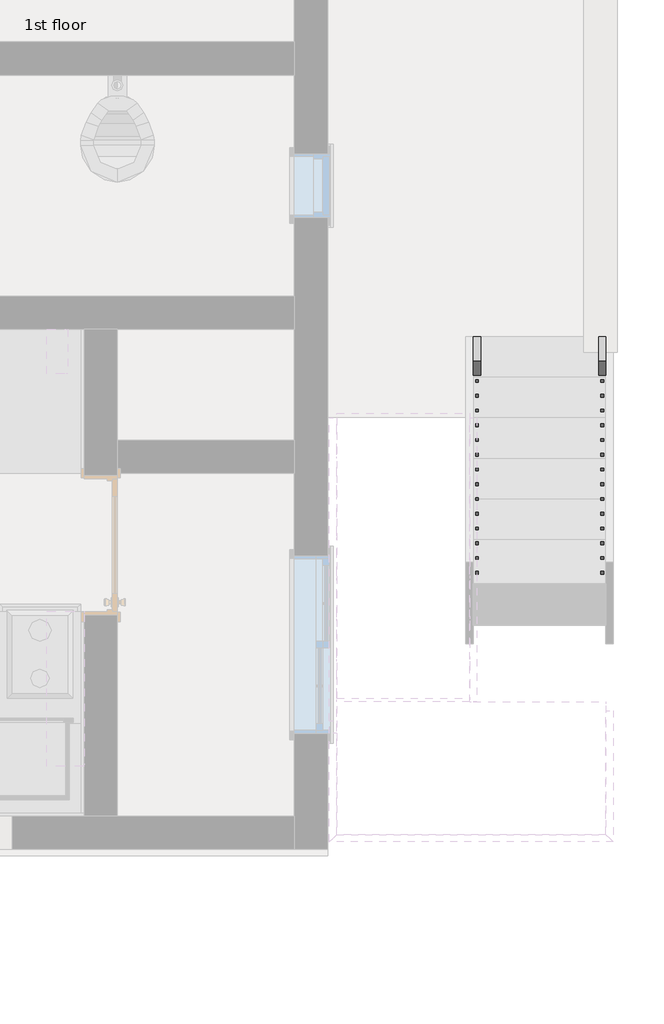
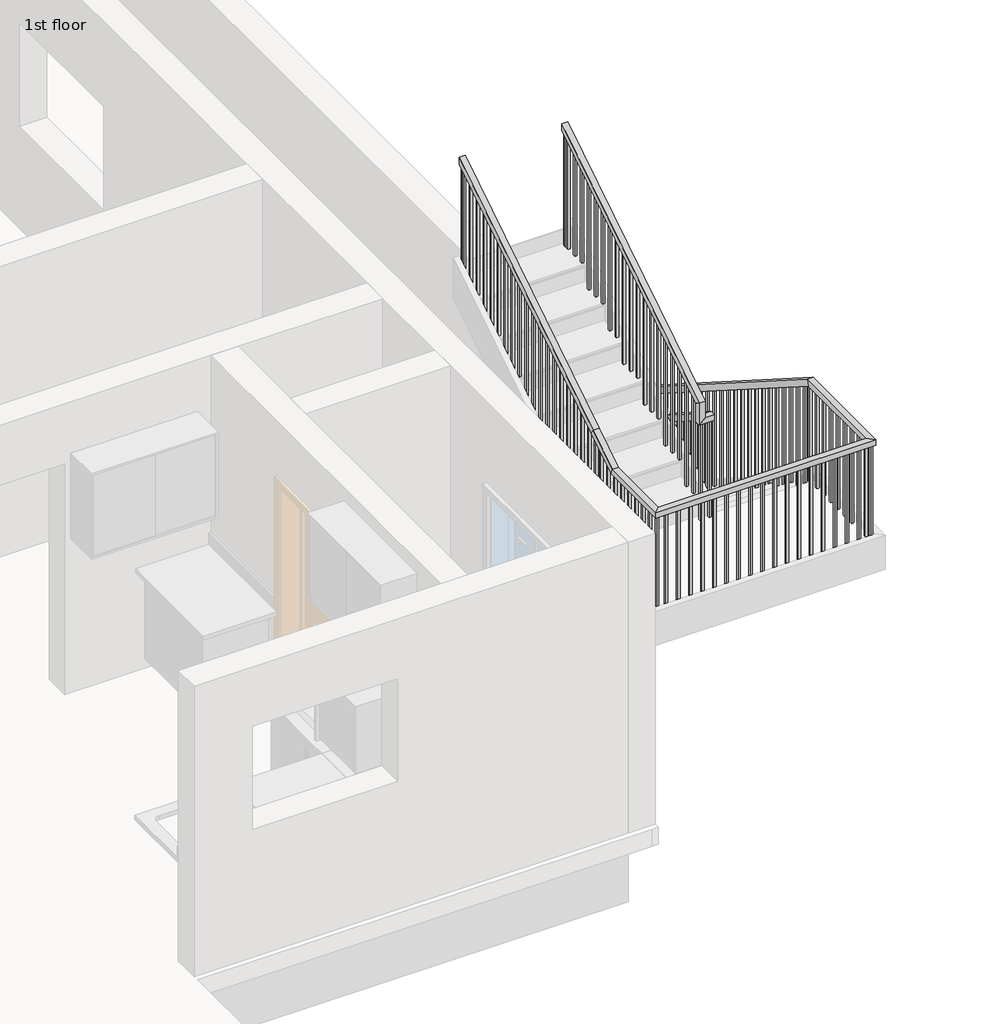
# One storey, part 6 of 8: 2 railings.
"""IFC4 building model written with IfcOpenShell, lengths in millimetres."""

from ifc_helpers import new_model, si_unit, frame, origin, place, context, project, spatial, polyline, outline, extrude, faceted_brep, element, save

model = new_model("IFC4")

# Units and contexts
model_context = context("Model", 3, world=origin())
ifc_project = project(units=[si_unit("LENGTHUNIT", "METRE", prefix="MILLI")], contexts=[model_context])

# Site, building, storey
site = spatial("IfcSite", under=ifc_project)
building = spatial("IfcBuilding", under=site)
storey = spatial("IfcBuildingStorey", under=building, Name="1st floor", Elevation=3810.0)

# Railings
placement = place(None, origin())
element("IfcRailing", 1, ObjectType="Handrail - Rectangular", at=placement, inside=storey, context=model_context, shape_type="SolidModel", body=[
    faceted_brep([(14287.3506237, -1074.7064015, 4902.2), (14287.3506237, -1074.7064015, 4841.986276), (14236.5506237, -1074.7064015, 4841.986276), (14236.5506237, -1074.7064015, 4902.2), (14287.3506237, -3589.3064015, 6502.4), (14236.5506237, -3589.3064015, 6502.4), (14236.5506237, -3589.3064015, 6442.186276), (14287.3506237, -3589.3064015, 6442.186276)], [[[0, 1, 2, 3]], [[4, 5, 6, 7]], [[1, 0, 4, 7]], [[2, 1, 7, 6]], [[3, 2, 6, 5]], [[0, 3, 5, 4]]]),
    faceted_brep([(14287.3506237, -3640.1064015, 6502.4), (14287.3506237, -3640.1064015, 6451.6), (14287.3506237, -3589.3064015, 6451.6), (14287.3506237, -3589.3064015, 6502.4), (14211.1506237, -3640.1064015, 6502.4), (14211.1506237, -3589.3064015, 6502.4), (14160.3506237, -3589.3064015, 6451.6), (14160.3506237, -3640.1064015, 6451.6)], [[[0, 1, 2, 3]], [[4, 5, 6, 7]], [[1, 0, 4, 7]], [[2, 1, 7, 6]], [[3, 2, 6, 5]], [[0, 3, 5, 4]]]),
    faceted_brep([(14211.1506237, -3640.1064015, 6502.4), (14160.3506237, -3640.1064015, 6451.6), (14160.3506237, -3589.3064015, 6451.6), (14211.1506237, -3589.3064015, 6502.4), (14211.1506237, -3640.1064015, 6647.8727273), (14211.1506237, -3589.3064015, 6619.986276), (14160.3506237, -3589.3064015, 6619.986276), (14160.3506237, -3640.1064015, 6647.8727273)], [[[0, 1, 2, 3]], [[4, 5, 6, 7]], [[1, 0, 4, 7]], [[2, 1, 7, 6]], [[3, 2, 6, 5]], [[0, 3, 5, 4]]]),
    faceted_brep([(14160.3506237, -3640.1064015, 6647.8727273), (14160.3506237, -3589.3064015, 6619.986276), (14211.1506237, -3589.3064015, 6619.986276), (14211.1506237, -3640.1064015, 6647.8727273), (14160.3506237, -1633.5064015, 7924.8), (14211.1506237, -1633.5064015, 7924.8), (14211.1506237, -1633.5064015, 7864.586276), (14160.3506237, -1633.5064015, 7864.586276)], [[[0, 1, 2, 3]], [[4, 5, 6, 7]], [[1, 0, 4, 7]], [[2, 1, 7, 6]], [[3, 2, 6, 5]], [[0, 3, 5, 4]]]),
    extrude(outline(polyline([(-1693.8314015, 7826.1976396), (-1674.7814015, 7838.3203669), (-1674.7814015, 6832.6), (-1693.8314015, 6832.6), (-1693.8314015, 7826.1976396)])), frame((14176.2256237, 0.0, 0.0), z_axis=(1.0, 0.0, 0.0), x_axis=(0.0, 1.0, 0.0)), (0.0, 0.0, 1.0), 19.05),
    extrude(outline(polyline([(-1795.4314015, 7761.5430941), (-1776.3814015, 7773.6658214), (-1776.3814015, 6832.6), (-1795.4314015, 6832.6), (-1795.4314015, 7761.5430941)])), frame((14176.2256237, 0.0, 0.0), z_axis=(1.0, 0.0, 0.0), x_axis=(0.0, 1.0, 0.0)), (0.0, 0.0, 1.0), 19.05),
    extrude(outline(polyline([(-1897.0314015, 7696.8885487), (-1877.9814015, 7709.011276), (-1877.9814015, 6832.6), (-1897.0314015, 6832.6), (-1897.0314015, 7696.8885487)])), frame((14176.2256237, 0.0, 0.0), z_axis=(1.0, 0.0, 0.0), x_axis=(0.0, 1.0, 0.0)), (0.0, 0.0, 1.0), 19.05),
    extrude(outline(polyline([(-1998.6314015, 7632.2340032), (-1979.5814015, 7644.3567305), (-1979.5814015, 6654.8), (-1998.6314015, 6654.8), (-1998.6314015, 7632.2340032)])), frame((14176.2256237, 0.0, 0.0), z_axis=(1.0, 0.0, 0.0), x_axis=(0.0, 1.0, 0.0)), (0.0, 0.0, 1.0), 19.05),
    extrude(outline(polyline([(-2100.2314015, 7567.5794578), (-2081.1814015, 7579.7021851), (-2081.1814015, 6654.8), (-2100.2314015, 6654.8), (-2100.2314015, 7567.5794578)])), frame((14176.2256237, 0.0, 0.0), z_axis=(1.0, 0.0, 0.0), x_axis=(0.0, 1.0, 0.0)), (0.0, 0.0, 1.0), 19.05),
    extrude(outline(polyline([(-2201.8314015, 7502.9249123), (-2182.7814015, 7515.0476396), (-2182.7814015, 6654.8), (-2201.8314015, 6654.8), (-2201.8314015, 7502.9249123)])), frame((14176.2256237, 0.0, 0.0), z_axis=(1.0, 0.0, 0.0), x_axis=(0.0, 1.0, 0.0)), (0.0, 0.0, 1.0), 19.05),
    extrude(outline(polyline([(-2303.4314015, 7438.2703669), (-2284.3814015, 7450.3930941), (-2284.3814015, 6477.0), (-2303.4314015, 6477.0), (-2303.4314015, 7438.2703669)])), frame((14176.2256237, 0.0, 0.0), z_axis=(1.0, 0.0, 0.0), x_axis=(0.0, 1.0, 0.0)), (0.0, 0.0, 1.0), 19.05),
    extrude(outline(polyline([(-2405.0314015, 7373.6158214), (-2385.9814015, 7385.7385487), (-2385.9814015, 6477.0), (-2405.0314015, 6477.0), (-2405.0314015, 7373.6158214)])), frame((14176.2256237, 0.0, 0.0), z_axis=(1.0, 0.0, 0.0), x_axis=(0.0, 1.0, 0.0)), (0.0, 0.0, 1.0), 19.05),
    extrude(outline(polyline([(-2506.6314015, 7308.961276), (-2487.5814015, 7321.0840032), (-2487.5814015, 6299.2), (-2506.6314015, 6299.2), (-2506.6314015, 7308.961276)])), frame((14176.2256237, 0.0, 0.0), z_axis=(1.0, 0.0, 0.0), x_axis=(0.0, 1.0, 0.0)), (0.0, 0.0, 1.0), 19.05),
    extrude(outline(polyline([(-2608.2314015, 7244.3067305), (-2589.1814015, 7256.4294578), (-2589.1814015, 6299.2), (-2608.2314015, 6299.2), (-2608.2314015, 7244.3067305)])), frame((14176.2256237, 0.0, 0.0), z_axis=(1.0, 0.0, 0.0), x_axis=(0.0, 1.0, 0.0)), (0.0, 0.0, 1.0), 19.05),
    extrude(outline(polyline([(-2709.8314015, 7179.6521851), (-2690.7814015, 7191.7749123), (-2690.7814015, 6299.2), (-2709.8314015, 6299.2), (-2709.8314015, 7179.6521851)])), frame((14176.2256237, 0.0, 0.0), z_axis=(1.0, 0.0, 0.0), x_axis=(0.0, 1.0, 0.0)), (0.0, 0.0, 1.0), 19.05),
    extrude(outline(polyline([(-2811.4314015, 7114.9976396), (-2792.3814015, 7127.1203669), (-2792.3814015, 6121.4), (-2811.4314015, 6121.4), (-2811.4314015, 7114.9976396)])), frame((14176.2256237, 0.0, 0.0), z_axis=(1.0, 0.0, 0.0), x_axis=(0.0, 1.0, 0.0)), (0.0, 0.0, 1.0), 19.05),
    extrude(outline(polyline([(-2913.0314015, 7050.3430941), (-2893.9814015, 7062.4658214), (-2893.9814015, 6121.4), (-2913.0314015, 6121.4), (-2913.0314015, 7050.3430941)])), frame((14176.2256237, 0.0, 0.0), z_axis=(1.0, 0.0, 0.0), x_axis=(0.0, 1.0, 0.0)), (0.0, 0.0, 1.0), 19.05),
    extrude(outline(polyline([(-3014.6314015, 6985.6885487), (-2995.5814015, 6997.811276), (-2995.5814015, 6121.4), (-3014.6314015, 6121.4), (-3014.6314015, 6985.6885487)])), frame((14176.2256237, 0.0, 0.0), z_axis=(1.0, 0.0, 0.0), x_axis=(0.0, 1.0, 0.0)), (0.0, 0.0, 1.0), 19.05),
    extrude(outline(polyline([(-3116.2314015, 6921.0340032), (-3097.1814015, 6933.1567305), (-3097.1814015, 5943.6), (-3116.2314015, 5943.6), (-3116.2314015, 6921.0340032)])), frame((14176.2256237, 0.0, 0.0), z_axis=(1.0, 0.0, 0.0), x_axis=(0.0, 1.0, 0.0)), (0.0, 0.0, 1.0), 19.05),
    extrude(outline(polyline([(-3217.8314015, 6856.3794578), (-3198.7814015, 6868.5021851), (-3198.7814015, 5943.6), (-3217.8314015, 5943.6), (-3217.8314015, 6856.3794578)])), frame((14176.2256237, 0.0, 0.0), z_axis=(1.0, 0.0, 0.0), x_axis=(0.0, 1.0, 0.0)), (0.0, 0.0, 1.0), 19.05),
    extrude(outline(polyline([(-3319.4314015, 6791.7249123), (-3300.3814015, 6803.8476396), (-3300.3814015, 5943.6), (-3319.4314015, 5943.6), (-3319.4314015, 6791.7249123)])), frame((14176.2256237, 0.0, 0.0), z_axis=(1.0, 0.0, 0.0), x_axis=(0.0, 1.0, 0.0)), (0.0, 0.0, 1.0), 19.05),
    extrude(outline(polyline([(-3421.0314015, 6727.0703669), (-3401.9814015, 6739.1930941), (-3401.9814015, 5765.8), (-3421.0314015, 5765.8), (-3421.0314015, 6727.0703669)])), frame((14176.2256237, 0.0, 0.0), z_axis=(1.0, 0.0, 0.0), x_axis=(0.0, 1.0, 0.0)), (0.0, 0.0, 1.0), 19.05),
    extrude(outline(polyline([(-3522.6314015, 6662.4158214), (-3503.5814015, 6674.5385487), (-3503.5814015, 5765.8), (-3522.6314015, 5765.8), (-3522.6314015, 6662.4158214)])), frame((14176.2256237, 0.0, 0.0), z_axis=(1.0, 0.0, 0.0), x_axis=(0.0, 1.0, 0.0)), (0.0, 0.0, 1.0), 19.05),
    extrude(outline(polyline([(-3522.6314015, 6399.7567305), (-3503.5814015, 6387.6340032), (-3503.5814015, 5410.2), (-3522.6314015, 5410.2), (-3522.6314015, 6399.7567305)])), frame((14252.4256237, 0.0, 0.0), z_axis=(1.0, 0.0, 0.0), x_axis=(0.0, 1.0, 0.0)), (0.0, 0.0, 1.0), 19.05),
    extrude(outline(polyline([(-3421.0314015, 6335.1021851), (-3401.9814015, 6322.9794578), (-3401.9814015, 5410.2), (-3421.0314015, 5410.2), (-3421.0314015, 6335.1021851)])), frame((14252.4256237, 0.0, 0.0), z_axis=(1.0, 0.0, 0.0), x_axis=(0.0, 1.0, 0.0)), (0.0, 0.0, 1.0), 19.05),
    extrude(outline(polyline([(-3319.4314015, 6270.4476396), (-3300.3814015, 6258.3249123), (-3300.3814015, 5410.2), (-3319.4314015, 5410.2), (-3319.4314015, 6270.4476396)])), frame((14252.4256237, 0.0, 0.0), z_axis=(1.0, 0.0, 0.0), x_axis=(0.0, 1.0, 0.0)), (0.0, 0.0, 1.0), 19.05),
    extrude(outline(polyline([(-3217.8314015, 6205.7930941), (-3198.7814015, 6193.6703669), (-3198.7814015, 5232.4), (-3217.8314015, 5232.4), (-3217.8314015, 6205.7930941)])), frame((14252.4256237, 0.0, 0.0), z_axis=(1.0, 0.0, 0.0), x_axis=(0.0, 1.0, 0.0)), (0.0, 0.0, 1.0), 19.05),
    extrude(outline(polyline([(-3116.2314015, 6141.1385487), (-3097.1814015, 6129.0158214), (-3097.1814015, 5232.4), (-3116.2314015, 5232.4), (-3116.2314015, 6141.1385487)])), frame((14252.4256237, 0.0, 0.0), z_axis=(1.0, 0.0, 0.0), x_axis=(0.0, 1.0, 0.0)), (0.0, 0.0, 1.0), 19.05),
    extrude(outline(polyline([(-3014.6314015, 6076.4840032), (-2995.5814015, 6064.361276), (-2995.5814015, 5054.6), (-3014.6314015, 5054.6), (-3014.6314015, 6076.4840032)])), frame((14252.4256237, 0.0, 0.0), z_axis=(1.0, 0.0, 0.0), x_axis=(0.0, 1.0, 0.0)), (0.0, 0.0, 1.0), 19.05),
    extrude(outline(polyline([(-2913.0314015, 6011.8294578), (-2893.9814015, 5999.7067305), (-2893.9814015, 5054.6), (-2913.0314015, 5054.6), (-2913.0314015, 6011.8294578)])), frame((14252.4256237, 0.0, 0.0), z_axis=(1.0, 0.0, 0.0), x_axis=(0.0, 1.0, 0.0)), (0.0, 0.0, 1.0), 19.05),
    extrude(outline(polyline([(-2811.4314015, 5947.1749123), (-2792.3814015, 5935.0521851), (-2792.3814015, 5054.6), (-2811.4314015, 5054.6), (-2811.4314015, 5947.1749123)])), frame((14252.4256237, 0.0, 0.0), z_axis=(1.0, 0.0, 0.0), x_axis=(0.0, 1.0, 0.0)), (0.0, 0.0, 1.0), 19.05),
    extrude(outline(polyline([(-2709.8314015, 5882.5203669), (-2690.7814015, 5870.3976396), (-2690.7814015, 4876.8), (-2709.8314015, 4876.8), (-2709.8314015, 5882.5203669)])), frame((14252.4256237, 0.0, 0.0), z_axis=(1.0, 0.0, 0.0), x_axis=(0.0, 1.0, 0.0)), (0.0, 0.0, 1.0), 19.05),
    extrude(outline(polyline([(-2608.2314015, 5817.8658214), (-2589.1814015, 5805.7430941), (-2589.1814015, 4876.8), (-2608.2314015, 4876.8), (-2608.2314015, 5817.8658214)])), frame((14252.4256237, 0.0, 0.0), z_axis=(1.0, 0.0, 0.0), x_axis=(0.0, 1.0, 0.0)), (0.0, 0.0, 1.0), 19.05),
    extrude(outline(polyline([(-2506.6314015, 5753.211276), (-2487.5814015, 5741.0885487), (-2487.5814015, 4876.8), (-2506.6314015, 4876.8), (-2506.6314015, 5753.211276)])), frame((14252.4256237, 0.0, 0.0), z_axis=(1.0, 0.0, 0.0), x_axis=(0.0, 1.0, 0.0)), (0.0, 0.0, 1.0), 19.05),
    extrude(outline(polyline([(-2405.0314015, 5688.5567305), (-2385.9814015, 5676.4340032), (-2385.9814015, 4699.0), (-2405.0314015, 4699.0), (-2405.0314015, 5688.5567305)])), frame((14252.4256237, 0.0, 0.0), z_axis=(1.0, 0.0, 0.0), x_axis=(0.0, 1.0, 0.0)), (0.0, 0.0, 1.0), 19.05),
    extrude(outline(polyline([(-2303.4314015, 5623.9021851), (-2284.3814015, 5611.7794578), (-2284.3814015, 4699.0), (-2303.4314015, 4699.0), (-2303.4314015, 5623.9021851)])), frame((14252.4256237, 0.0, 0.0), z_axis=(1.0, 0.0, 0.0), x_axis=(0.0, 1.0, 0.0)), (0.0, 0.0, 1.0), 19.05),
    extrude(outline(polyline([(-2201.8314015, 5559.2476396), (-2182.7814015, 5547.1249123), (-2182.7814015, 4699.0), (-2201.8314015, 4699.0), (-2201.8314015, 5559.2476396)])), frame((14252.4256237, 0.0, 0.0), z_axis=(1.0, 0.0, 0.0), x_axis=(0.0, 1.0, 0.0)), (0.0, 0.0, 1.0), 19.05),
    extrude(outline(polyline([(-2100.2314015, 5494.5930941), (-2081.1814015, 5482.4703669), (-2081.1814015, 4521.2), (-2100.2314015, 4521.2), (-2100.2314015, 5494.5930941)])), frame((14252.4256237, 0.0, 0.0), z_axis=(1.0, 0.0, 0.0), x_axis=(0.0, 1.0, 0.0)), (0.0, 0.0, 1.0), 19.05),
    extrude(outline(polyline([(-1998.6314015, 5429.9385487), (-1979.5814015, 5417.8158214), (-1979.5814015, 4521.2), (-1998.6314015, 4521.2), (-1998.6314015, 5429.9385487)])), frame((14252.4256237, 0.0, 0.0), z_axis=(1.0, 0.0, 0.0), x_axis=(0.0, 1.0, 0.0)), (0.0, 0.0, 1.0), 19.05),
    extrude(outline(polyline([(-1897.0314015, 5365.2840032), (-1877.9814015, 5353.161276), (-1877.9814015, 4343.4), (-1897.0314015, 4343.4), (-1897.0314015, 5365.2840032)])), frame((14252.4256237, 0.0, 0.0), z_axis=(1.0, 0.0, 0.0), x_axis=(0.0, 1.0, 0.0)), (0.0, 0.0, 1.0), 19.05),
    extrude(outline(polyline([(-1795.4314015, 5300.6294578), (-1776.3814015, 5288.5067305), (-1776.3814015, 4343.4), (-1795.4314015, 4343.4), (-1795.4314015, 5300.6294578)])), frame((14252.4256237, 0.0, 0.0), z_axis=(1.0, 0.0, 0.0), x_axis=(0.0, 1.0, 0.0)), (0.0, 0.0, 1.0), 19.05),
    extrude(outline(polyline([(-1693.8314015, 5235.9749123), (-1674.7814015, 5223.8521851), (-1674.7814015, 4343.4), (-1693.8314015, 4343.4), (-1693.8314015, 5235.9749123)])), frame((14252.4256237, 0.0, 0.0), z_axis=(1.0, 0.0, 0.0), x_axis=(0.0, 1.0, 0.0)), (0.0, 0.0, 1.0), 19.05),
    extrude(outline(polyline([(-1592.2314015, 5171.3203669), (-1573.1814015, 5159.1976396), (-1573.1814015, 4165.6), (-1592.2314015, 4165.6), (-1592.2314015, 5171.3203669)])), frame((14252.4256237, 0.0, 0.0), z_axis=(1.0, 0.0, 0.0), x_axis=(0.0, 1.0, 0.0)), (0.0, 0.0, 1.0), 19.05),
    extrude(outline(polyline([(-1490.6314015, 5106.6658214), (-1471.5814015, 5094.5430941), (-1471.5814015, 4165.6), (-1490.6314015, 4165.6), (-1490.6314015, 5106.6658214)])), frame((14252.4256237, 0.0, 0.0), z_axis=(1.0, 0.0, 0.0), x_axis=(0.0, 1.0, 0.0)), (0.0, 0.0, 1.0), 19.05),
    extrude(outline(polyline([(-1389.0314015, 5042.011276), (-1369.9814015, 5029.8885487), (-1369.9814015, 4165.6), (-1389.0314015, 4165.6), (-1389.0314015, 5042.011276)])), frame((14252.4256237, 0.0, 0.0), z_axis=(1.0, 0.0, 0.0), x_axis=(0.0, 1.0, 0.0)), (0.0, 0.0, 1.0), 19.05),
    extrude(outline(polyline([(-1287.4314015, 4977.3567305), (-1268.3814015, 4965.2340032), (-1268.3814015, 3987.8), (-1287.4314015, 3987.8), (-1287.4314015, 4977.3567305)])), frame((14252.4256237, 0.0, 0.0), z_axis=(1.0, 0.0, 0.0), x_axis=(0.0, 1.0, 0.0)), (0.0, 0.0, 1.0), 19.05),
    extrude(outline(polyline([(-1185.8314015, 4912.7021851), (-1166.7814015, 4900.5794578), (-1166.7814015, 3987.8), (-1185.8314015, 3987.8), (-1185.8314015, 4912.7021851)])), frame((14252.4256237, 0.0, 0.0), z_axis=(1.0, 0.0, 0.0), x_axis=(0.0, 1.0, 0.0)), (0.0, 0.0, 1.0), 19.05),
    extrude(outline(polyline([(14195.2756237, -3605.1814015), (14195.2756237, -3624.2314015), (14176.2256237, -3624.2314015), (14176.2256237, -3605.1814015), (14195.2756237, -3605.1814015)])), frame((0.0, 0.0, 5588.0), z_axis=(0.0, 0.0, 1.0), x_axis=(1.0, 0.0, 0.0)), (0.0, 0.0, 1.0), 863.6),
    extrude(outline(polyline([(-3624.2314015, 6464.411276), (-3605.1814015, 6452.2885487), (-3605.1814015, 5588.0), (-3624.2314015, 5588.0), (-3624.2314015, 6464.411276)])), frame((14252.4256237, 0.0, 0.0), z_axis=(1.0, 0.0, 0.0), x_axis=(0.0, 1.0, 0.0)), (0.0, 0.0, 1.0), 19.05),
    extrude(outline(polyline([(-1652.5564015, 7852.4635487), (-1633.5064015, 7864.586276), (-1633.5064015, 6832.6), (-1652.5564015, 6832.6), (-1652.5564015, 7852.4635487)])), frame((14176.2256237, 0.0, 0.0), z_axis=(1.0, 0.0, 0.0), x_axis=(0.0, 1.0, 0.0)), (0.0, 0.0, 1.0), 19.05),
    extrude(outline(polyline([(-1093.7564015, 4854.1090032), (-1074.7064015, 4841.986276), (-1074.7064015, 3987.8), (-1093.7564015, 3987.8), (-1093.7564015, 4854.1090032)])), frame((14252.4256237, 0.0, 0.0), z_axis=(1.0, 0.0, 0.0), x_axis=(0.0, 1.0, 0.0)), (0.0, 0.0, 1.0), 19.05),
])
element("IfcRailing", 2, ObjectType="Handrail - Rectangular", at=placement, inside=storey, context=model_context, shape_type="SolidModel", body=[
    faceted_brep([(15150.9506237, -1074.7064015, 4902.2), (15150.9506237, -1074.7064015, 4841.986276), (15100.1506237, -1074.7064015, 4841.986276), (15100.1506237, -1074.7064015, 4902.2), (15150.9506237, -3589.3064015, 6502.4), (15150.9506237, -3604.0993964, 6451.6), (15100.1506237, -3604.0993964, 6451.6), (15100.1506237, -3589.3064015, 6502.4), (15150.9506237, -4503.7064015, 6502.4), (15150.9506237, -4503.7064015, 6451.6), (15100.1506237, -4452.9064015, 6451.6), (15100.1506237, -4452.9064015, 6502.4), (13296.7506237, -4503.7064015, 6502.4), (13296.7506237, -4503.7064015, 6451.6), (13347.5506237, -4452.9064015, 6451.6), (13347.5506237, -4452.9064015, 6502.4), (13296.7506237, -3868.7064015, 6502.4), (13296.7506237, -3853.9134066, 6451.6), (13347.5506237, -3853.9134066, 6451.6), (13347.5506237, -3868.7064015, 6502.4), (13296.7506237, -3589.3064015, 6680.2), (13296.7506237, -3562.0331265, 6637.3419964), (13347.5506237, -3562.0331265, 6637.3419964), (13347.5506237, -3589.3064015, 6680.2), (13296.7506237, -1633.5064015, 7924.8), (13347.5506237, -1633.5064015, 7924.8), (13347.5506237, -1633.5064015, 7864.586276), (13296.7506237, -1633.5064015, 7864.586276)], [[[0, 1, 2, 3]], [[1, 0, 4, 5]], [[2, 1, 5, 6]], [[3, 2, 6, 7]], [[0, 3, 7, 4]], [[5, 4, 8, 9]], [[6, 5, 9, 10]], [[7, 6, 10, 11]], [[4, 7, 11, 8]], [[9, 8, 12, 13]], [[10, 9, 13, 14]], [[11, 10, 14, 15]], [[8, 11, 15, 12]], [[13, 12, 16, 17]], [[14, 13, 17, 18]], [[15, 14, 18, 19]], [[12, 15, 19, 16]], [[17, 16, 20, 21]], [[18, 17, 21, 22]], [[19, 18, 22, 23]], [[16, 19, 23, 20]], [[24, 25, 26, 27]], [[21, 20, 24, 27]], [[22, 21, 27, 26]], [[23, 22, 26, 25]], [[20, 23, 25, 24]]]),
    extrude(outline(polyline([(-1649.3814015, 7854.4840032), (-1649.3814015, 6832.6), (-1668.4314015, 6832.6), (-1668.4314015, 7842.361276), (-1649.3814015, 7854.4840032)])), frame((13312.6256237, 0.0, 0.0), z_axis=(1.0, 0.0, 0.0), x_axis=(0.0, 1.0, 0.0)), (0.0, 0.0, 1.0), 19.05),
    extrude(outline(polyline([(-1750.9814015, 7789.8294578), (-1750.9814015, 6832.6), (-1770.0314015, 6832.6), (-1770.0314015, 7777.7067305), (-1750.9814015, 7789.8294578)])), frame((13312.6256237, 0.0, 0.0), z_axis=(1.0, 0.0, 0.0), x_axis=(0.0, 1.0, 0.0)), (0.0, 0.0, 1.0), 19.05),
    extrude(outline(polyline([(-1852.5814015, 7725.1749123), (-1852.5814015, 6832.6), (-1871.6314015, 6832.6), (-1871.6314015, 7713.0521851), (-1852.5814015, 7725.1749123)])), frame((13312.6256237, 0.0, 0.0), z_axis=(1.0, 0.0, 0.0), x_axis=(0.0, 1.0, 0.0)), (0.0, 0.0, 1.0), 19.05),
    extrude(outline(polyline([(-1954.1814015, 7660.5203669), (-1954.1814015, 6654.8), (-1973.2314015, 6654.8), (-1973.2314015, 7648.3976396), (-1954.1814015, 7660.5203669)])), frame((13312.6256237, 0.0, 0.0), z_axis=(1.0, 0.0, 0.0), x_axis=(0.0, 1.0, 0.0)), (0.0, 0.0, 1.0), 19.05),
    extrude(outline(polyline([(-2055.7814015, 7595.8658214), (-2055.7814015, 6654.8), (-2074.8314015, 6654.8), (-2074.8314015, 7583.7430941), (-2055.7814015, 7595.8658214)])), frame((13312.6256237, 0.0, 0.0), z_axis=(1.0, 0.0, 0.0), x_axis=(0.0, 1.0, 0.0)), (0.0, 0.0, 1.0), 19.05),
    extrude(outline(polyline([(-2157.3814015, 7531.211276), (-2157.3814015, 6654.8), (-2176.4314015, 6654.8), (-2176.4314015, 7519.0885487), (-2157.3814015, 7531.211276)])), frame((13312.6256237, 0.0, 0.0), z_axis=(1.0, 0.0, 0.0), x_axis=(0.0, 1.0, 0.0)), (0.0, 0.0, 1.0), 19.05),
    extrude(outline(polyline([(-2258.9814015, 7466.5567305), (-2258.9814015, 6477.0), (-2278.0314015, 6477.0), (-2278.0314015, 7454.4340032), (-2258.9814015, 7466.5567305)])), frame((13312.6256237, 0.0, 0.0), z_axis=(1.0, 0.0, 0.0), x_axis=(0.0, 1.0, 0.0)), (0.0, 0.0, 1.0), 19.05),
    extrude(outline(polyline([(-2360.5814015, 7401.9021851), (-2360.5814015, 6477.0), (-2379.6314015, 6477.0), (-2379.6314015, 7389.7794578), (-2360.5814015, 7401.9021851)])), frame((13312.6256237, 0.0, 0.0), z_axis=(1.0, 0.0, 0.0), x_axis=(0.0, 1.0, 0.0)), (0.0, 0.0, 1.0), 19.05),
    extrude(outline(polyline([(-2462.1814015, 7337.2476396), (-2462.1814015, 6477.0), (-2481.2314015, 6477.0), (-2481.2314015, 7325.1249123), (-2462.1814015, 7337.2476396)])), frame((13312.6256237, 0.0, 0.0), z_axis=(1.0, 0.0, 0.0), x_axis=(0.0, 1.0, 0.0)), (0.0, 0.0, 1.0), 19.05),
    extrude(outline(polyline([(-2563.7814015, 7272.5930941), (-2563.7814015, 6299.2), (-2582.8314015, 6299.2), (-2582.8314015, 7260.4703669), (-2563.7814015, 7272.5930941)])), frame((13312.6256237, 0.0, 0.0), z_axis=(1.0, 0.0, 0.0), x_axis=(0.0, 1.0, 0.0)), (0.0, 0.0, 1.0), 19.05),
    extrude(outline(polyline([(-2665.3814015, 7207.9385487), (-2665.3814015, 6299.2), (-2684.4314015, 6299.2), (-2684.4314015, 7195.8158214), (-2665.3814015, 7207.9385487)])), frame((13312.6256237, 0.0, 0.0), z_axis=(1.0, 0.0, 0.0), x_axis=(0.0, 1.0, 0.0)), (0.0, 0.0, 1.0), 19.05),
    extrude(outline(polyline([(-2766.9814015, 7143.2840032), (-2766.9814015, 6121.4), (-2786.0314015, 6121.4), (-2786.0314015, 7131.161276), (-2766.9814015, 7143.2840032)])), frame((13312.6256237, 0.0, 0.0), z_axis=(1.0, 0.0, 0.0), x_axis=(0.0, 1.0, 0.0)), (0.0, 0.0, 1.0), 19.05),
    extrude(outline(polyline([(-2868.5814015, 7078.6294578), (-2868.5814015, 6121.4), (-2887.6314015, 6121.4), (-2887.6314015, 7066.5067305), (-2868.5814015, 7078.6294578)])), frame((13312.6256237, 0.0, 0.0), z_axis=(1.0, 0.0, 0.0), x_axis=(0.0, 1.0, 0.0)), (0.0, 0.0, 1.0), 19.05),
    extrude(outline(polyline([(-2970.1814015, 7013.9749123), (-2970.1814015, 6121.4), (-2989.2314015, 6121.4), (-2989.2314015, 7001.8521851), (-2970.1814015, 7013.9749123)])), frame((13312.6256237, 0.0, 0.0), z_axis=(1.0, 0.0, 0.0), x_axis=(0.0, 1.0, 0.0)), (0.0, 0.0, 1.0), 19.05),
    extrude(outline(polyline([(-3071.7814015, 6949.3203669), (-3071.7814015, 5943.6), (-3090.8314015, 5943.6), (-3090.8314015, 6937.1976396), (-3071.7814015, 6949.3203669)])), frame((13312.6256237, 0.0, 0.0), z_axis=(1.0, 0.0, 0.0), x_axis=(0.0, 1.0, 0.0)), (0.0, 0.0, 1.0), 19.05),
    extrude(outline(polyline([(-3173.3814015, 6884.6658214), (-3173.3814015, 5943.6), (-3192.4314015, 5943.6), (-3192.4314015, 6872.5430941), (-3173.3814015, 6884.6658214)])), frame((13312.6256237, 0.0, 0.0), z_axis=(1.0, 0.0, 0.0), x_axis=(0.0, 1.0, 0.0)), (0.0, 0.0, 1.0), 19.05),
    extrude(outline(polyline([(-3274.9814015, 6820.011276), (-3274.9814015, 5943.6), (-3294.0314015, 5943.6), (-3294.0314015, 6807.8885487), (-3274.9814015, 6820.011276)])), frame((13312.6256237, 0.0, 0.0), z_axis=(1.0, 0.0, 0.0), x_axis=(0.0, 1.0, 0.0)), (0.0, 0.0, 1.0), 19.05),
    extrude(outline(polyline([(-3376.5814015, 6755.3567305), (-3376.5814015, 5765.8), (-3395.6314015, 5765.8), (-3395.6314015, 6743.2340032), (-3376.5814015, 6755.3567305)])), frame((13312.6256237, 0.0, 0.0), z_axis=(1.0, 0.0, 0.0), x_axis=(0.0, 1.0, 0.0)), (0.0, 0.0, 1.0), 19.05),
    extrude(outline(polyline([(-3478.1814015, 6690.7021851), (-3478.1814015, 5765.8), (-3497.2314015, 5765.8), (-3497.2314015, 6678.5794578), (-3478.1814015, 6690.7021851)])), frame((13312.6256237, 0.0, 0.0), z_axis=(1.0, 0.0, 0.0), x_axis=(0.0, 1.0, 0.0)), (0.0, 0.0, 1.0), 19.05),
    extrude(outline(polyline([(-3655.9814015, 6577.5567305), (-3655.9814015, 5588.0), (-3675.0314015, 5588.0), (-3675.0314015, 6565.4340032), (-3655.9814015, 6577.5567305)])), frame((13312.6256237, 0.0, 0.0), z_axis=(1.0, 0.0, 0.0), x_axis=(0.0, 1.0, 0.0)), (0.0, 0.0, 1.0), 19.05),
    extrude(outline(polyline([(-3757.5814015, 6512.9021851), (-3757.5814015, 5588.0), (-3776.6314015, 5588.0), (-3776.6314015, 6500.7794578), (-3757.5814015, 6512.9021851)])), frame((13312.6256237, 0.0, 0.0), z_axis=(1.0, 0.0, 0.0), x_axis=(0.0, 1.0, 0.0)), (0.0, 0.0, 1.0), 19.05),
    extrude(outline(polyline([(13312.6256237, -3878.2314015), (13312.6256237, -3859.1814015), (13331.6756237, -3859.1814015), (13331.6756237, -3878.2314015), (13312.6256237, -3878.2314015)])), frame((0.0, 0.0, 5588.0), z_axis=(0.0, 0.0, 1.0), x_axis=(1.0, 0.0, 0.0)), (0.0, 0.0, 1.0), 863.6),
    extrude(outline(polyline([(13312.6256237, -3979.8314015), (13312.6256237, -3960.7814015), (13331.6756237, -3960.7814015), (13331.6756237, -3979.8314015), (13312.6256237, -3979.8314015)])), frame((0.0, 0.0, 5588.0), z_axis=(0.0, 0.0, 1.0), x_axis=(1.0, 0.0, 0.0)), (0.0, 0.0, 1.0), 863.6),
    extrude(outline(polyline([(13312.6256237, -4081.4314015), (13312.6256237, -4062.3814015), (13331.6756237, -4062.3814015), (13331.6756237, -4081.4314015), (13312.6256237, -4081.4314015)])), frame((0.0, 0.0, 5588.0), z_axis=(0.0, 0.0, 1.0), x_axis=(1.0, 0.0, 0.0)), (0.0, 0.0, 1.0), 863.6),
    extrude(outline(polyline([(13312.6256237, -4183.0314015), (13312.6256237, -4163.9814015), (13331.6756237, -4163.9814015), (13331.6756237, -4183.0314015), (13312.6256237, -4183.0314015)])), frame((0.0, 0.0, 5588.0), z_axis=(0.0, 0.0, 1.0), x_axis=(1.0, 0.0, 0.0)), (0.0, 0.0, 1.0), 863.6),
    extrude(outline(polyline([(13312.6256237, -4284.6314015), (13312.6256237, -4265.5814015), (13331.6756237, -4265.5814015), (13331.6756237, -4284.6314015), (13312.6256237, -4284.6314015)])), frame((0.0, 0.0, 5588.0), z_axis=(0.0, 0.0, 1.0), x_axis=(1.0, 0.0, 0.0)), (0.0, 0.0, 1.0), 863.6),
    extrude(outline(polyline([(13312.6256237, -4386.2314015), (13312.6256237, -4367.1814015), (13331.6756237, -4367.1814015), (13331.6756237, -4386.2314015), (13312.6256237, -4386.2314015)])), frame((0.0, 0.0, 5588.0), z_axis=(0.0, 0.0, 1.0), x_axis=(1.0, 0.0, 0.0)), (0.0, 0.0, 1.0), 863.6),
    extrude(outline(polyline([(13407.8756237, -4487.8314015), (13388.8256237, -4487.8314015), (13388.8256237, -4468.7814015), (13407.8756237, -4468.7814015), (13407.8756237, -4487.8314015)])), frame((0.0, 0.0, 5588.0), z_axis=(0.0, 0.0, 1.0), x_axis=(1.0, 0.0, 0.0)), (0.0, 0.0, 1.0), 863.6),
    extrude(outline(polyline([(13509.4756237, -4487.8314015), (13490.4256237, -4487.8314015), (13490.4256237, -4468.7814015), (13509.4756237, -4468.7814015), (13509.4756237, -4487.8314015)])), frame((0.0, 0.0, 5588.0), z_axis=(0.0, 0.0, 1.0), x_axis=(1.0, 0.0, 0.0)), (0.0, 0.0, 1.0), 863.6),
    extrude(outline(polyline([(13611.0756237, -4487.8314015), (13592.0256237, -4487.8314015), (13592.0256237, -4468.7814015), (13611.0756237, -4468.7814015), (13611.0756237, -4487.8314015)])), frame((0.0, 0.0, 5588.0), z_axis=(0.0, 0.0, 1.0), x_axis=(1.0, 0.0, 0.0)), (0.0, 0.0, 1.0), 863.6),
    extrude(outline(polyline([(13712.6756237, -4487.8314015), (13693.6256237, -4487.8314015), (13693.6256237, -4468.7814015), (13712.6756237, -4468.7814015), (13712.6756237, -4487.8314015)])), frame((0.0, 0.0, 5588.0), z_axis=(0.0, 0.0, 1.0), x_axis=(1.0, 0.0, 0.0)), (0.0, 0.0, 1.0), 863.6),
    extrude(outline(polyline([(13814.2756237, -4487.8314015), (13795.2256237, -4487.8314015), (13795.2256237, -4468.7814015), (13814.2756237, -4468.7814015), (13814.2756237, -4487.8314015)])), frame((0.0, 0.0, 5588.0), z_axis=(0.0, 0.0, 1.0), x_axis=(1.0, 0.0, 0.0)), (0.0, 0.0, 1.0), 863.6),
    extrude(outline(polyline([(13915.8756237, -4487.8314015), (13896.8256237, -4487.8314015), (13896.8256237, -4468.7814015), (13915.8756237, -4468.7814015), (13915.8756237, -4487.8314015)])), frame((0.0, 0.0, 5588.0), z_axis=(0.0, 0.0, 1.0), x_axis=(1.0, 0.0, 0.0)), (0.0, 0.0, 1.0), 863.6),
    extrude(outline(polyline([(14017.4756237, -4487.8314015), (13998.4256237, -4487.8314015), (13998.4256237, -4468.7814015), (14017.4756237, -4468.7814015), (14017.4756237, -4487.8314015)])), frame((0.0, 0.0, 5588.0), z_axis=(0.0, 0.0, 1.0), x_axis=(1.0, 0.0, 0.0)), (0.0, 0.0, 1.0), 863.6),
    extrude(outline(polyline([(14119.0756237, -4487.8314015), (14100.0256237, -4487.8314015), (14100.0256237, -4468.7814015), (14119.0756237, -4468.7814015), (14119.0756237, -4487.8314015)])), frame((0.0, 0.0, 5588.0), z_axis=(0.0, 0.0, 1.0), x_axis=(1.0, 0.0, 0.0)), (0.0, 0.0, 1.0), 863.6),
    extrude(outline(polyline([(14220.6756237, -4487.8314015), (14201.6256237, -4487.8314015), (14201.6256237, -4468.7814015), (14220.6756237, -4468.7814015), (14220.6756237, -4487.8314015)])), frame((0.0, 0.0, 5588.0), z_axis=(0.0, 0.0, 1.0), x_axis=(1.0, 0.0, 0.0)), (0.0, 0.0, 1.0), 863.6),
    extrude(outline(polyline([(14322.2756237, -4487.8314015), (14303.2256237, -4487.8314015), (14303.2256237, -4468.7814015), (14322.2756237, -4468.7814015), (14322.2756237, -4487.8314015)])), frame((0.0, 0.0, 5588.0), z_axis=(0.0, 0.0, 1.0), x_axis=(1.0, 0.0, 0.0)), (0.0, 0.0, 1.0), 863.6),
    extrude(outline(polyline([(14423.8756237, -4487.8314015), (14404.8256237, -4487.8314015), (14404.8256237, -4468.7814015), (14423.8756237, -4468.7814015), (14423.8756237, -4487.8314015)])), frame((0.0, 0.0, 5588.0), z_axis=(0.0, 0.0, 1.0), x_axis=(1.0, 0.0, 0.0)), (0.0, 0.0, 1.0), 863.6),
    extrude(outline(polyline([(14525.4756237, -4487.8314015), (14506.4256237, -4487.8314015), (14506.4256237, -4468.7814015), (14525.4756237, -4468.7814015), (14525.4756237, -4487.8314015)])), frame((0.0, 0.0, 5588.0), z_axis=(0.0, 0.0, 1.0), x_axis=(1.0, 0.0, 0.0)), (0.0, 0.0, 1.0), 863.6),
    extrude(outline(polyline([(14627.0756237, -4487.8314015), (14608.0256237, -4487.8314015), (14608.0256237, -4468.7814015), (14627.0756237, -4468.7814015), (14627.0756237, -4487.8314015)])), frame((0.0, 0.0, 5588.0), z_axis=(0.0, 0.0, 1.0), x_axis=(1.0, 0.0, 0.0)), (0.0, 0.0, 1.0), 863.6),
    extrude(outline(polyline([(14728.6756237, -4487.8314015), (14709.6256237, -4487.8314015), (14709.6256237, -4468.7814015), (14728.6756237, -4468.7814015), (14728.6756237, -4487.8314015)])), frame((0.0, 0.0, 5588.0), z_axis=(0.0, 0.0, 1.0), x_axis=(1.0, 0.0, 0.0)), (0.0, 0.0, 1.0), 863.6),
    extrude(outline(polyline([(14830.2756237, -4487.8314015), (14811.2256237, -4487.8314015), (14811.2256237, -4468.7814015), (14830.2756237, -4468.7814015), (14830.2756237, -4487.8314015)])), frame((0.0, 0.0, 5588.0), z_axis=(0.0, 0.0, 1.0), x_axis=(1.0, 0.0, 0.0)), (0.0, 0.0, 1.0), 863.6),
    extrude(outline(polyline([(14931.8756237, -4487.8314015), (14912.8256237, -4487.8314015), (14912.8256237, -4468.7814015), (14931.8756237, -4468.7814015), (14931.8756237, -4487.8314015)])), frame((0.0, 0.0, 5588.0), z_axis=(0.0, 0.0, 1.0), x_axis=(1.0, 0.0, 0.0)), (0.0, 0.0, 1.0), 863.6),
    extrude(outline(polyline([(15033.4756237, -4487.8314015), (15014.4256237, -4487.8314015), (15014.4256237, -4468.7814015), (15033.4756237, -4468.7814015), (15033.4756237, -4487.8314015)])), frame((0.0, 0.0, 5588.0), z_axis=(0.0, 0.0, 1.0), x_axis=(1.0, 0.0, 0.0)), (0.0, 0.0, 1.0), 863.6),
    extrude(outline(polyline([(15135.0756237, -4392.5814015), (15135.0756237, -4411.6314015), (15116.0256237, -4411.6314015), (15116.0256237, -4392.5814015), (15135.0756237, -4392.5814015)])), frame((0.0, 0.0, 5588.0), z_axis=(0.0, 0.0, 1.0), x_axis=(1.0, 0.0, 0.0)), (0.0, 0.0, 1.0), 863.6),
    extrude(outline(polyline([(15135.0756237, -4290.9814015), (15135.0756237, -4310.0314015), (15116.0256237, -4310.0314015), (15116.0256237, -4290.9814015), (15135.0756237, -4290.9814015)])), frame((0.0, 0.0, 5588.0), z_axis=(0.0, 0.0, 1.0), x_axis=(1.0, 0.0, 0.0)), (0.0, 0.0, 1.0), 863.6),
    extrude(outline(polyline([(15135.0756237, -4189.3814015), (15135.0756237, -4208.4314015), (15116.0256237, -4208.4314015), (15116.0256237, -4189.3814015), (15135.0756237, -4189.3814015)])), frame((0.0, 0.0, 5588.0), z_axis=(0.0, 0.0, 1.0), x_axis=(1.0, 0.0, 0.0)), (0.0, 0.0, 1.0), 863.6),
    extrude(outline(polyline([(15135.0756237, -4087.7814015), (15135.0756237, -4106.8314015), (15116.0256237, -4106.8314015), (15116.0256237, -4087.7814015), (15135.0756237, -4087.7814015)])), frame((0.0, 0.0, 5588.0), z_axis=(0.0, 0.0, 1.0), x_axis=(1.0, 0.0, 0.0)), (0.0, 0.0, 1.0), 863.6),
    extrude(outline(polyline([(15135.0756237, -3986.1814015), (15135.0756237, -4005.2314015), (15116.0256237, -4005.2314015), (15116.0256237, -3986.1814015), (15135.0756237, -3986.1814015)])), frame((0.0, 0.0, 5588.0), z_axis=(0.0, 0.0, 1.0), x_axis=(1.0, 0.0, 0.0)), (0.0, 0.0, 1.0), 863.6),
    extrude(outline(polyline([(15135.0756237, -3884.5814015), (15135.0756237, -3903.6314015), (15116.0256237, -3903.6314015), (15116.0256237, -3884.5814015), (15135.0756237, -3884.5814015)])), frame((0.0, 0.0, 5588.0), z_axis=(0.0, 0.0, 1.0), x_axis=(1.0, 0.0, 0.0)), (0.0, 0.0, 1.0), 863.6),
    extrude(outline(polyline([(15135.0756237, -3782.9814015), (15135.0756237, -3802.0314015), (15116.0256237, -3802.0314015), (15116.0256237, -3782.9814015), (15135.0756237, -3782.9814015)])), frame((0.0, 0.0, 5588.0), z_axis=(0.0, 0.0, 1.0), x_axis=(1.0, 0.0, 0.0)), (0.0, 0.0, 1.0), 863.6),
    extrude(outline(polyline([(15135.0756237, -3681.3814015), (15135.0756237, -3700.4314015), (15116.0256237, -3700.4314015), (15116.0256237, -3681.3814015), (15135.0756237, -3681.3814015)])), frame((0.0, 0.0, 5588.0), z_axis=(0.0, 0.0, 1.0), x_axis=(1.0, 0.0, 0.0)), (0.0, 0.0, 1.0), 863.6),
    extrude(outline(polyline([(-3503.5814015, 6387.6340032), (-3503.5814015, 5410.2), (-3522.6314015, 5410.2), (-3522.6314015, 6399.7567305), (-3503.5814015, 6387.6340032)])), frame((15116.0256237, 0.0, 0.0), z_axis=(1.0, 0.0, 0.0), x_axis=(0.0, 1.0, 0.0)), (0.0, 0.0, 1.0), 19.05),
    extrude(outline(polyline([(-3401.9814015, 6322.9794578), (-3401.9814015, 5410.2), (-3421.0314015, 5410.2), (-3421.0314015, 6335.1021851), (-3401.9814015, 6322.9794578)])), frame((15116.0256237, 0.0, 0.0), z_axis=(1.0, 0.0, 0.0), x_axis=(0.0, 1.0, 0.0)), (0.0, 0.0, 1.0), 19.05),
    extrude(outline(polyline([(-3300.3814015, 6258.3249123), (-3300.3814015, 5410.2), (-3319.4314015, 5410.2), (-3319.4314015, 6270.4476396), (-3300.3814015, 6258.3249123)])), frame((15116.0256237, 0.0, 0.0), z_axis=(1.0, 0.0, 0.0), x_axis=(0.0, 1.0, 0.0)), (0.0, 0.0, 1.0), 19.05),
    extrude(outline(polyline([(-3198.7814015, 6193.6703669), (-3198.7814015, 5232.4), (-3217.8314015, 5232.4), (-3217.8314015, 6205.7930941), (-3198.7814015, 6193.6703669)])), frame((15116.0256237, 0.0, 0.0), z_axis=(1.0, 0.0, 0.0), x_axis=(0.0, 1.0, 0.0)), (0.0, 0.0, 1.0), 19.05),
    extrude(outline(polyline([(-3097.1814015, 6129.0158214), (-3097.1814015, 5232.4), (-3116.2314015, 5232.4), (-3116.2314015, 6141.1385487), (-3097.1814015, 6129.0158214)])), frame((15116.0256237, 0.0, 0.0), z_axis=(1.0, 0.0, 0.0), x_axis=(0.0, 1.0, 0.0)), (0.0, 0.0, 1.0), 19.05),
    extrude(outline(polyline([(-2995.5814015, 6064.361276), (-2995.5814015, 5054.6), (-3014.6314015, 5054.6), (-3014.6314015, 6076.4840032), (-2995.5814015, 6064.361276)])), frame((15116.0256237, 0.0, 0.0), z_axis=(1.0, 0.0, 0.0), x_axis=(0.0, 1.0, 0.0)), (0.0, 0.0, 1.0), 19.05),
    extrude(outline(polyline([(-2893.9814015, 5999.7067305), (-2893.9814015, 5054.6), (-2913.0314015, 5054.6), (-2913.0314015, 6011.8294578), (-2893.9814015, 5999.7067305)])), frame((15116.0256237, 0.0, 0.0), z_axis=(1.0, 0.0, 0.0), x_axis=(0.0, 1.0, 0.0)), (0.0, 0.0, 1.0), 19.05),
    extrude(outline(polyline([(-2792.3814015, 5935.0521851), (-2792.3814015, 5054.6), (-2811.4314015, 5054.6), (-2811.4314015, 5947.1749123), (-2792.3814015, 5935.0521851)])), frame((15116.0256237, 0.0, 0.0), z_axis=(1.0, 0.0, 0.0), x_axis=(0.0, 1.0, 0.0)), (0.0, 0.0, 1.0), 19.05),
    extrude(outline(polyline([(-2690.7814015, 5870.3976396), (-2690.7814015, 4876.8), (-2709.8314015, 4876.8), (-2709.8314015, 5882.5203669), (-2690.7814015, 5870.3976396)])), frame((15116.0256237, 0.0, 0.0), z_axis=(1.0, 0.0, 0.0), x_axis=(0.0, 1.0, 0.0)), (0.0, 0.0, 1.0), 19.05),
    extrude(outline(polyline([(-2589.1814015, 5805.7430941), (-2589.1814015, 4876.8), (-2608.2314015, 4876.8), (-2608.2314015, 5817.8658214), (-2589.1814015, 5805.7430941)])), frame((15116.0256237, 0.0, 0.0), z_axis=(1.0, 0.0, 0.0), x_axis=(0.0, 1.0, 0.0)), (0.0, 0.0, 1.0), 19.05),
    extrude(outline(polyline([(-2487.5814015, 5741.0885487), (-2487.5814015, 4876.8), (-2506.6314015, 4876.8), (-2506.6314015, 5753.211276), (-2487.5814015, 5741.0885487)])), frame((15116.0256237, 0.0, 0.0), z_axis=(1.0, 0.0, 0.0), x_axis=(0.0, 1.0, 0.0)), (0.0, 0.0, 1.0), 19.05),
    extrude(outline(polyline([(-2385.9814015, 5676.4340032), (-2385.9814015, 4699.0), (-2405.0314015, 4699.0), (-2405.0314015, 5688.5567305), (-2385.9814015, 5676.4340032)])), frame((15116.0256237, 0.0, 0.0), z_axis=(1.0, 0.0, 0.0), x_axis=(0.0, 1.0, 0.0)), (0.0, 0.0, 1.0), 19.05),
    extrude(outline(polyline([(-2284.3814015, 5611.7794578), (-2284.3814015, 4699.0), (-2303.4314015, 4699.0), (-2303.4314015, 5623.9021851), (-2284.3814015, 5611.7794578)])), frame((15116.0256237, 0.0, 0.0), z_axis=(1.0, 0.0, 0.0), x_axis=(0.0, 1.0, 0.0)), (0.0, 0.0, 1.0), 19.05),
    extrude(outline(polyline([(-2182.7814015, 5547.1249123), (-2182.7814015, 4699.0), (-2201.8314015, 4699.0), (-2201.8314015, 5559.2476396), (-2182.7814015, 5547.1249123)])), frame((15116.0256237, 0.0, 0.0), z_axis=(1.0, 0.0, 0.0), x_axis=(0.0, 1.0, 0.0)), (0.0, 0.0, 1.0), 19.05),
    extrude(outline(polyline([(-2081.1814015, 5482.4703669), (-2081.1814015, 4521.2), (-2100.2314015, 4521.2), (-2100.2314015, 5494.5930941), (-2081.1814015, 5482.4703669)])), frame((15116.0256237, 0.0, 0.0), z_axis=(1.0, 0.0, 0.0), x_axis=(0.0, 1.0, 0.0)), (0.0, 0.0, 1.0), 19.05),
    extrude(outline(polyline([(-1979.5814015, 5417.8158214), (-1979.5814015, 4521.2), (-1998.6314015, 4521.2), (-1998.6314015, 5429.9385487), (-1979.5814015, 5417.8158214)])), frame((15116.0256237, 0.0, 0.0), z_axis=(1.0, 0.0, 0.0), x_axis=(0.0, 1.0, 0.0)), (0.0, 0.0, 1.0), 19.05),
    extrude(outline(polyline([(-1877.9814015, 5353.161276), (-1877.9814015, 4343.4), (-1897.0314015, 4343.4), (-1897.0314015, 5365.2840032), (-1877.9814015, 5353.161276)])), frame((15116.0256237, 0.0, 0.0), z_axis=(1.0, 0.0, 0.0), x_axis=(0.0, 1.0, 0.0)), (0.0, 0.0, 1.0), 19.05),
    extrude(outline(polyline([(-1776.3814015, 5288.5067305), (-1776.3814015, 4343.4), (-1795.4314015, 4343.4), (-1795.4314015, 5300.6294578), (-1776.3814015, 5288.5067305)])), frame((15116.0256237, 0.0, 0.0), z_axis=(1.0, 0.0, 0.0), x_axis=(0.0, 1.0, 0.0)), (0.0, 0.0, 1.0), 19.05),
    extrude(outline(polyline([(-1674.7814015, 5223.8521851), (-1674.7814015, 4343.4), (-1693.8314015, 4343.4), (-1693.8314015, 5235.9749123), (-1674.7814015, 5223.8521851)])), frame((15116.0256237, 0.0, 0.0), z_axis=(1.0, 0.0, 0.0), x_axis=(0.0, 1.0, 0.0)), (0.0, 0.0, 1.0), 19.05),
    extrude(outline(polyline([(-1573.1814015, 5159.1976396), (-1573.1814015, 4165.6), (-1592.2314015, 4165.6), (-1592.2314015, 5171.3203669), (-1573.1814015, 5159.1976396)])), frame((15116.0256237, 0.0, 0.0), z_axis=(1.0, 0.0, 0.0), x_axis=(0.0, 1.0, 0.0)), (0.0, 0.0, 1.0), 19.05),
    extrude(outline(polyline([(-1471.5814015, 5094.5430941), (-1471.5814015, 4165.6), (-1490.6314015, 4165.6), (-1490.6314015, 5106.6658214), (-1471.5814015, 5094.5430941)])), frame((15116.0256237, 0.0, 0.0), z_axis=(1.0, 0.0, 0.0), x_axis=(0.0, 1.0, 0.0)), (0.0, 0.0, 1.0), 19.05),
    extrude(outline(polyline([(-1369.9814015, 5029.8885487), (-1369.9814015, 4165.6), (-1389.0314015, 4165.6), (-1389.0314015, 5042.011276), (-1369.9814015, 5029.8885487)])), frame((15116.0256237, 0.0, 0.0), z_axis=(1.0, 0.0, 0.0), x_axis=(0.0, 1.0, 0.0)), (0.0, 0.0, 1.0), 19.05),
    extrude(outline(polyline([(-1268.3814015, 4965.2340032), (-1268.3814015, 3987.8), (-1287.4314015, 3987.8), (-1287.4314015, 4977.3567305), (-1268.3814015, 4965.2340032)])), frame((15116.0256237, 0.0, 0.0), z_axis=(1.0, 0.0, 0.0), x_axis=(0.0, 1.0, 0.0)), (0.0, 0.0, 1.0), 19.05),
    extrude(outline(polyline([(-1166.7814015, 4900.5794578), (-1166.7814015, 3987.8), (-1185.8314015, 3987.8), (-1185.8314015, 4912.7021851), (-1166.7814015, 4900.5794578)])), frame((15116.0256237, 0.0, 0.0), z_axis=(1.0, 0.0, 0.0), x_axis=(0.0, 1.0, 0.0)), (0.0, 0.0, 1.0), 19.05),
    extrude(outline(polyline([(-3579.7814015, 6626.0476396), (-3579.7814015, 5588.0), (-3598.8314015, 5588.0), (-3598.8314015, 6613.9249123), (-3579.7814015, 6626.0476396)])), frame((13312.6256237, 0.0, 0.0), z_axis=(1.0, 0.0, 0.0), x_axis=(0.0, 1.0, 0.0)), (0.0, 0.0, 1.0), 19.05),
    extrude(outline(polyline([(13331.6756237, -4487.8314015), (13312.6256237, -4487.8314015), (13312.6256237, -4468.7814015), (13331.6756237, -4468.7814015), (13331.6756237, -4487.8314015)])), frame((0.0, 0.0, 5588.0), z_axis=(0.0, 0.0, 1.0), x_axis=(1.0, 0.0, 0.0)), (0.0, 0.0, 1.0), 863.6),
    extrude(outline(polyline([(15135.0756237, -4468.7814015), (15135.0756237, -4487.8314015), (15116.0256237, -4487.8314015), (15116.0256237, -4468.7814015), (15135.0756237, -4468.7814015)])), frame((0.0, 0.0, 5588.0), z_axis=(0.0, 0.0, 1.0), x_axis=(1.0, 0.0, 0.0)), (0.0, 0.0, 1.0), 863.6),
    extrude(outline(polyline([(-3579.7814015, 6436.1249123), (-3579.7814015, 5588.0), (-3598.8314015, 5588.0), (-3598.8314015, 6448.2476396), (-3579.7814015, 6436.1249123)])), frame((15116.0256237, 0.0, 0.0), z_axis=(1.0, 0.0, 0.0), x_axis=(0.0, 1.0, 0.0)), (0.0, 0.0, 1.0), 19.05),
    extrude(outline(polyline([(-1633.5064015, 7864.586276), (-1633.5064015, 6832.6), (-1652.5564015, 6832.6), (-1652.5564015, 7852.4635487), (-1633.5064015, 7864.586276)])), frame((13312.6256237, 0.0, 0.0), z_axis=(1.0, 0.0, 0.0), x_axis=(0.0, 1.0, 0.0)), (0.0, 0.0, 1.0), 19.05),
    extrude(outline(polyline([(-1074.7064015, 4841.986276), (-1074.7064015, 3987.8), (-1093.7564015, 3987.8), (-1093.7564015, 4854.1090032), (-1074.7064015, 4841.986276)])), frame((15116.0256237, 0.0, 0.0), z_axis=(1.0, 0.0, 0.0), x_axis=(0.0, 1.0, 0.0)), (0.0, 0.0, 1.0), 19.05),
])

save(model, "model.ifc")

# Revit data of these elements
# Type "Handrail - Rectangular"
#   Assembly Code = "C2010400"
#   built-in parameter 1008612 = 0.0416667 (stored number, unit not read)
#   built-in parameter 1008611 = 0.0416667 (stored number, unit not read)
#   built-in parameter 1008609 = 0.333333 (stored number, unit not read)
#   built-in parameter 1008604 = 0.166667 (stored number, unit not read)
#   built-in parameter 1008603 = 0.166667 (stored number, unit not read)
#   Railing Height = 3' - 0"
#   built-in parameter 1008630 = 2
#   built-in parameter 1008610 = 2
#   built-in parameter 1008618 = Baluster - Square : 3/4"
# Elements 1, 2 (IfcRailing, "Handrail - Rectangular")
#   Phase Created = New Construction
